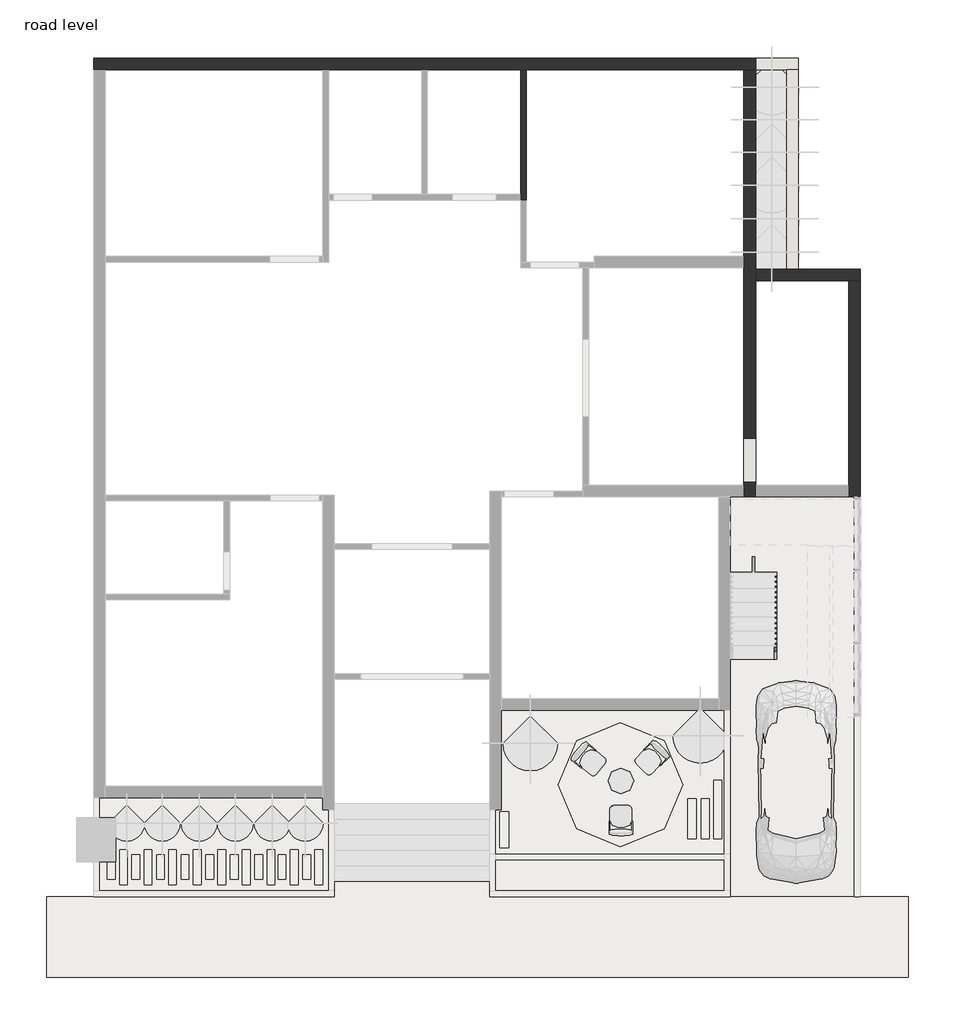
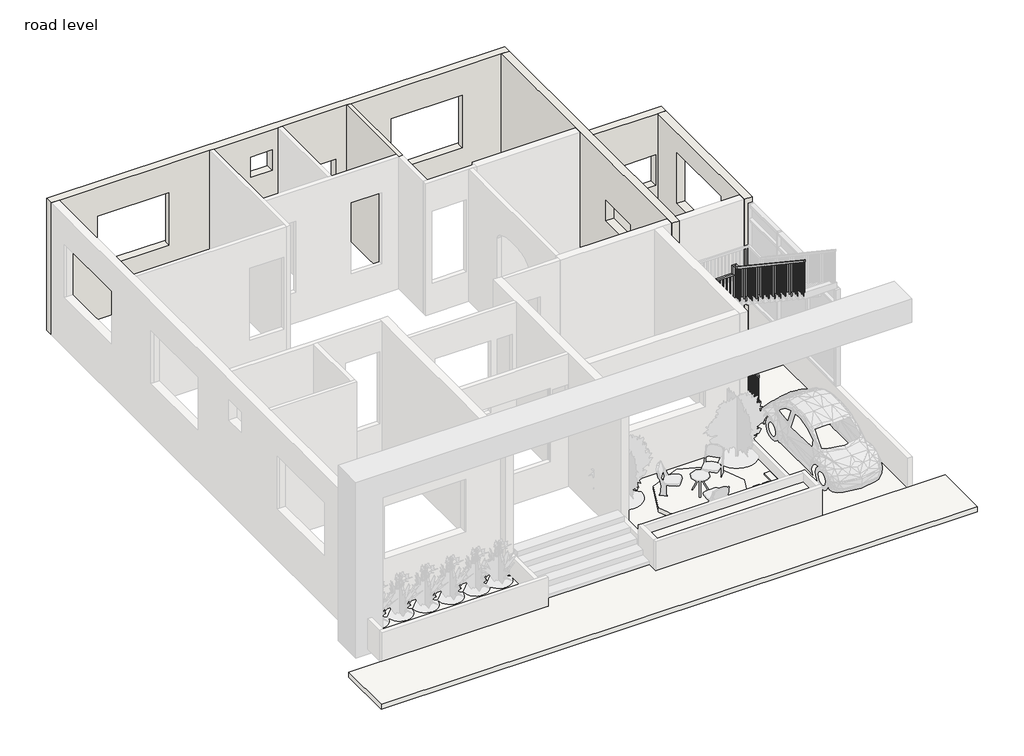
# One storey, part 2 of 3: 9 slabs, 7 walls, 1 railing.
"""IFC4 building model written with IfcOpenShell, lengths in millimetres."""

from ifc_helpers import new_model, si_unit, point, frame, frame_2d, origin, origin_with_axes, place, context, project, spatial, polyline, circle_curve, trimmed, segment, composite_curve, outline, extrude, faceted_brep, element, save

model = new_model("IFC4")

# Units and contexts
model_context = context("Model", 3, world=origin())
ifc_project = project(units=[si_unit("LENGTHUNIT", "METRE", prefix="MILLI")], contexts=[model_context])

# Site, building, storey
site = spatial("IfcSite", under=ifc_project)
building = spatial("IfcBuilding", under=site)
storey = spatial("IfcBuildingStorey", under=building, Name="road level", Elevation=0.0)

# Railing
placement = place(None, origin())
element("IfcRailing", 1, ObjectType="Handrail - Rectangular", at=placement, inside=storey, context=model_context, shape_type="SolidModel", body=[
    faceted_brep([(-6809.0994093, 3499.0237487, 1101.4363636), (-6809.0994093, 3499.0237487, 1040.3046237), (-6758.2994093, 3499.0237487, 1040.3046237), (-6758.2994093, 3499.0237487, 1101.4363636), (-6809.0994093, 5658.0237487, 2546.7173554), (-6809.0994093, 5708.8237487, 2519.592227), (-6758.2994093, 5708.8237487, 2519.592227), (-6758.2994093, 5658.0237487, 2546.7173554), (-6809.0994093, 5658.0237487, 2597.7272727), (-6809.0994093, 5708.8237487, 2546.9272727), (-6758.2994093, 5708.8237487, 2546.9272727), (-6758.2994093, 5658.0237487, 2597.7272727), (-6809.0994093, 5785.0237487, 2597.7272727), (-6809.0994093, 5785.0237487, 2546.9272727), (-6758.2994093, 5734.2237487, 2546.9272727), (-6758.2994093, 5734.2237487, 2597.7272727), (-6682.0994093, 5785.0237487, 2597.7272727), (-6682.0994093, 5785.0237487, 2546.9272727), (-6682.0994093, 5734.2237487, 2546.9272727), (-6682.0994093, 5734.2237487, 2597.7272727), (-6224.8994093, 5785.0237487, 2597.7272727), (-6174.0994093, 5785.0237487, 2546.9272727), (-6174.0994093, 5734.2237487, 2546.9272727), (-6224.8994093, 5734.2237487, 2597.7272727), (-6224.8994093, 5785.0237487, 2835.7735537), (-6174.0994093, 5785.0237487, 2784.9735537), (-6174.0994093, 5734.2237487, 2784.9735537), (-6224.8994093, 5734.2237487, 2835.7735537), (-6097.8994093, 5785.0237487, 2835.7735537), (-6097.8994093, 5785.0237487, 2784.9735537), (-6148.6994093, 5734.2237487, 2784.9735537), (-6148.6994093, 5734.2237487, 2835.7735537), (-6097.8994093, 5658.0237487, 2835.7735537), (-6097.8994093, 5642.5899149, 2784.9735537), (-6148.6994093, 5642.5899149, 2784.9735537), (-6148.6994093, 5658.0237487, 2835.7735537), (-6097.8994093, 2381.4237487, 5029.2), (-6148.6994093, 2381.4237487, 5029.2), (-6148.6994093, 2381.4237487, 4968.06826), (-6097.8994093, 2381.4237487, 4968.06826)], [[[0, 1, 2, 3]], [[1, 0, 4, 5]], [[2, 1, 5, 6]], [[3, 2, 6, 7]], [[0, 3, 7, 4]], [[5, 4, 8, 9]], [[6, 5, 9, 10]], [[7, 6, 10, 11]], [[4, 7, 11, 8]], [[9, 8, 12, 13]], [[10, 9, 13, 14]], [[11, 10, 14, 15]], [[8, 11, 15, 12]], [[13, 12, 16, 17]], [[14, 13, 17, 18]], [[15, 14, 18, 19]], [[12, 15, 19, 16]], [[17, 16, 20, 21]], [[18, 17, 21, 22]], [[19, 18, 22, 23]], [[16, 19, 23, 20]], [[21, 20, 24, 25]], [[22, 21, 25, 26]], [[23, 22, 26, 27]], [[20, 23, 27, 24]], [[25, 24, 28, 29]], [[26, 25, 29, 30]], [[27, 26, 30, 31]], [[24, 27, 31, 28]], [[29, 28, 32, 33]], [[30, 29, 33, 34]], [[31, 30, 34, 35]], [[28, 31, 35, 32]], [[36, 37, 38, 39]], [[33, 32, 36, 39]], [[34, 33, 39, 38]], [[35, 34, 38, 37]], [[32, 35, 37, 36]]]),
    extrude(outline(polyline([(2397.2987487, 4957.4411939), (2416.3487487, 4944.6887146), (2416.3487487, 3927.7636364), (2397.2987487, 3927.7636364), (2397.2987487, 4957.4411939)])), frame((-6132.8244093, 0.0, 0.0), z_axis=(1.0, 0.0, 0.0), x_axis=(0.0, 1.0, 0.0)), (0.0, 0.0, 1.0), 19.05),
    extrude(outline(polyline([(2498.8987487, 4889.4279708), (2517.9487487, 4876.6754914), (2517.9487487, 3927.7636364), (2498.8987487, 3927.7636364), (2498.8987487, 4889.4279708)])), frame((-6132.8244093, 0.0, 0.0), z_axis=(1.0, 0.0, 0.0), x_axis=(0.0, 1.0, 0.0)), (0.0, 0.0, 1.0), 19.05),
    extrude(outline(polyline([(2600.4987487, 4821.4147476), (2619.5487487, 4808.6622683), (2619.5487487, 3927.7636364), (2600.4987487, 3927.7636364), (2600.4987487, 4821.4147476)])), frame((-6132.8244093, 0.0, 0.0), z_axis=(1.0, 0.0, 0.0), x_axis=(0.0, 1.0, 0.0)), (0.0, 0.0, 1.0), 19.05),
    extrude(outline(polyline([(2702.0987487, 4753.4015245), (2721.1487487, 4740.6490452), (2721.1487487, 3740.7272727), (2702.0987487, 3740.7272727), (2702.0987487, 4753.4015245)])), frame((-6132.8244093, 0.0, 0.0), z_axis=(1.0, 0.0, 0.0), x_axis=(0.0, 1.0, 0.0)), (0.0, 0.0, 1.0), 19.05),
    extrude(outline(polyline([(2803.6987487, 4685.3883014), (2822.7487487, 4672.635822), (2822.7487487, 3740.7272727), (2803.6987487, 3740.7272727), (2803.6987487, 4685.3883014)])), frame((-6132.8244093, 0.0, 0.0), z_axis=(1.0, 0.0, 0.0), x_axis=(0.0, 1.0, 0.0)), (0.0, 0.0, 1.0), 19.05),
    extrude(outline(polyline([(2905.2987487, 4617.3750782), (2924.3487487, 4604.6225989), (2924.3487487, 3740.7272727), (2905.2987487, 3740.7272727), (2905.2987487, 4617.3750782)])), frame((-6132.8244093, 0.0, 0.0), z_axis=(1.0, 0.0, 0.0), x_axis=(0.0, 1.0, 0.0)), (0.0, 0.0, 1.0), 19.05),
    extrude(outline(polyline([(3006.8987487, 4549.3618551), (3025.9487487, 4536.6093757), (3025.9487487, 3553.6909091), (3006.8987487, 3553.6909091), (3006.8987487, 4549.3618551)])), frame((-6132.8244093, 0.0, 0.0), z_axis=(1.0, 0.0, 0.0), x_axis=(0.0, 1.0, 0.0)), (0.0, 0.0, 1.0), 19.05),
    extrude(outline(polyline([(3108.4987487, 4481.3486319), (3127.5487487, 4468.5961526), (3127.5487487, 3553.6909091), (3108.4987487, 3553.6909091), (3108.4987487, 4481.3486319)])), frame((-6132.8244093, 0.0, 0.0), z_axis=(1.0, 0.0, 0.0), x_axis=(0.0, 1.0, 0.0)), (0.0, 0.0, 1.0), 19.05),
    extrude(outline(polyline([(3210.0987487, 4413.3354088), (3229.1487487, 4400.5829295), (3229.1487487, 3553.6909091), (3210.0987487, 3553.6909091), (3210.0987487, 4413.3354088)])), frame((-6132.8244093, 0.0, 0.0), z_axis=(1.0, 0.0, 0.0), x_axis=(0.0, 1.0, 0.0)), (0.0, 0.0, 1.0), 19.05),
    extrude(outline(polyline([(3311.6987487, 4345.3221857), (3330.7487487, 4332.5697063), (3330.7487487, 3366.6545455), (3311.6987487, 3366.6545455), (3311.6987487, 4345.3221857)])), frame((-6132.8244093, 0.0, 0.0), z_axis=(1.0, 0.0, 0.0), x_axis=(0.0, 1.0, 0.0)), (0.0, 0.0, 1.0), 19.05),
    extrude(outline(polyline([(3413.2987487, 4277.3089625), (3432.3487487, 4264.5564832), (3432.3487487, 3366.6545455), (3413.2987487, 3366.6545455), (3413.2987487, 4277.3089625)])), frame((-6132.8244093, 0.0, 0.0), z_axis=(1.0, 0.0, 0.0), x_axis=(0.0, 1.0, 0.0)), (0.0, 0.0, 1.0), 19.05),
    extrude(outline(polyline([(3514.8987487, 4209.2957394), (3533.9487487, 4196.54326), (3533.9487487, 3179.6181818), (3514.8987487, 3179.6181818), (3514.8987487, 4209.2957394)])), frame((-6132.8244093, 0.0, 0.0), z_axis=(1.0, 0.0, 0.0), x_axis=(0.0, 1.0, 0.0)), (0.0, 0.0, 1.0), 19.05),
    extrude(outline(polyline([(3616.4987487, 4141.2825162), (3635.5487487, 4128.5300369), (3635.5487487, 3179.6181818), (3616.4987487, 3179.6181818), (3616.4987487, 4141.2825162)])), frame((-6132.8244093, 0.0, 0.0), z_axis=(1.0, 0.0, 0.0), x_axis=(0.0, 1.0, 0.0)), (0.0, 0.0, 1.0), 19.05),
    extrude(outline(polyline([(3718.0987487, 4073.2692931), (3737.1487487, 4060.5168138), (3737.1487487, 3179.6181818), (3718.0987487, 3179.6181818), (3718.0987487, 4073.2692931)])), frame((-6132.8244093, 0.0, 0.0), z_axis=(1.0, 0.0, 0.0), x_axis=(0.0, 1.0, 0.0)), (0.0, 0.0, 1.0), 19.05),
    extrude(outline(polyline([(3819.6987487, 4005.25607), (3838.7487487, 3992.5035906), (3838.7487487, 2992.5818182), (3819.6987487, 2992.5818182), (3819.6987487, 4005.25607)])), frame((-6132.8244093, 0.0, 0.0), z_axis=(1.0, 0.0, 0.0), x_axis=(0.0, 1.0, 0.0)), (0.0, 0.0, 1.0), 19.05),
    extrude(outline(polyline([(3921.2987487, 3937.2428468), (3940.3487487, 3924.4903675), (3940.3487487, 2992.5818182), (3921.2987487, 2992.5818182), (3921.2987487, 3937.2428468)])), frame((-6132.8244093, 0.0, 0.0), z_axis=(1.0, 0.0, 0.0), x_axis=(0.0, 1.0, 0.0)), (0.0, 0.0, 1.0), 19.05),
    extrude(outline(polyline([(4022.8987487, 3869.2296237), (4041.9487487, 3856.4771443), (4041.9487487, 2992.5818182), (4022.8987487, 2992.5818182), (4022.8987487, 3869.2296237)])), frame((-6132.8244093, 0.0, 0.0), z_axis=(1.0, 0.0, 0.0), x_axis=(0.0, 1.0, 0.0)), (0.0, 0.0, 1.0), 19.05),
    extrude(outline(polyline([(4124.4987487, 3801.2164005), (4143.5487487, 3788.4639212), (4143.5487487, 2805.5454545), (4124.4987487, 2805.5454545), (4124.4987487, 3801.2164005)])), frame((-6132.8244093, 0.0, 0.0), z_axis=(1.0, 0.0, 0.0), x_axis=(0.0, 1.0, 0.0)), (0.0, 0.0, 1.0), 19.05),
    extrude(outline(polyline([(4226.0987487, 3733.2031774), (4245.1487487, 3720.4506981), (4245.1487487, 2805.5454545), (4226.0987487, 2805.5454545), (4226.0987487, 3733.2031774)])), frame((-6132.8244093, 0.0, 0.0), z_axis=(1.0, 0.0, 0.0), x_axis=(0.0, 1.0, 0.0)), (0.0, 0.0, 1.0), 19.05),
    extrude(outline(polyline([(4327.6987487, 3665.1899543), (4346.7487487, 3652.4374749), (4346.7487487, 2805.5454545), (4327.6987487, 2805.5454545), (4327.6987487, 3665.1899543)])), frame((-6132.8244093, 0.0, 0.0), z_axis=(1.0, 0.0, 0.0), x_axis=(0.0, 1.0, 0.0)), (0.0, 0.0, 1.0), 19.05),
    extrude(outline(polyline([(4429.2987487, 3597.1767311), (4448.3487487, 3584.4242518), (4448.3487487, 2618.5090909), (4429.2987487, 2618.5090909), (4429.2987487, 3597.1767311)])), frame((-6132.8244093, 0.0, 0.0), z_axis=(1.0, 0.0, 0.0), x_axis=(0.0, 1.0, 0.0)), (0.0, 0.0, 1.0), 19.05),
    extrude(outline(polyline([(4530.8987487, 3529.163508), (4549.9487487, 3516.4110286), (4549.9487487, 2618.5090909), (4530.8987487, 2618.5090909), (4530.8987487, 3529.163508)])), frame((-6132.8244093, 0.0, 0.0), z_axis=(1.0, 0.0, 0.0), x_axis=(0.0, 1.0, 0.0)), (0.0, 0.0, 1.0), 19.05),
    extrude(outline(polyline([(4632.4987487, 3461.1502848), (4651.5487487, 3448.3978055), (4651.5487487, 2431.4727273), (4632.4987487, 2431.4727273), (4632.4987487, 3461.1502848)])), frame((-6132.8244093, 0.0, 0.0), z_axis=(1.0, 0.0, 0.0), x_axis=(0.0, 1.0, 0.0)), (0.0, 0.0, 1.0), 19.05),
    extrude(outline(polyline([(4734.0987487, 3393.1370617), (4753.1487487, 3380.3845824), (4753.1487487, 2431.4727273), (4734.0987487, 2431.4727273), (4734.0987487, 3393.1370617)])), frame((-6132.8244093, 0.0, 0.0), z_axis=(1.0, 0.0, 0.0), x_axis=(0.0, 1.0, 0.0)), (0.0, 0.0, 1.0), 19.05),
    extrude(outline(polyline([(4835.6987487, 3325.1238386), (4854.7487487, 3312.3713592), (4854.7487487, 2431.4727273), (4835.6987487, 2431.4727273), (4835.6987487, 3325.1238386)])), frame((-6132.8244093, 0.0, 0.0), z_axis=(1.0, 0.0, 0.0), x_axis=(0.0, 1.0, 0.0)), (0.0, 0.0, 1.0), 19.05),
    extrude(outline(polyline([(4937.2987487, 3257.1106154), (4956.3487487, 3244.3581361), (4956.3487487, 2244.4363636), (4937.2987487, 2244.4363636), (4937.2987487, 3257.1106154)])), frame((-6132.8244093, 0.0, 0.0), z_axis=(1.0, 0.0, 0.0), x_axis=(0.0, 1.0, 0.0)), (0.0, 0.0, 1.0), 19.05),
    extrude(outline(polyline([(5038.8987487, 3189.0973923), (5057.9487487, 3176.3449129), (5057.9487487, 2244.4363636), (5038.8987487, 2244.4363636), (5038.8987487, 3189.0973923)])), frame((-6132.8244093, 0.0, 0.0), z_axis=(1.0, 0.0, 0.0), x_axis=(0.0, 1.0, 0.0)), (0.0, 0.0, 1.0), 19.05),
    extrude(outline(polyline([(5140.4987487, 3121.0841691), (5159.5487487, 3108.3316898), (5159.5487487, 2244.4363636), (5140.4987487, 2244.4363636), (5140.4987487, 3121.0841691)])), frame((-6132.8244093, 0.0, 0.0), z_axis=(1.0, 0.0, 0.0), x_axis=(0.0, 1.0, 0.0)), (0.0, 0.0, 1.0), 19.05),
    extrude(outline(polyline([(5242.0987487, 3053.070946), (5261.1487487, 3040.3184667), (5261.1487487, 2057.4), (5242.0987487, 2057.4), (5242.0987487, 3053.070946)])), frame((-6132.8244093, 0.0, 0.0), z_axis=(1.0, 0.0, 0.0), x_axis=(0.0, 1.0, 0.0)), (0.0, 0.0, 1.0), 19.05),
    extrude(outline(polyline([(5343.6987487, 2985.0577229), (5362.7487487, 2972.3052435), (5362.7487487, 2057.4), (5343.6987487, 2057.4), (5343.6987487, 2985.0577229)])), frame((-6132.8244093, 0.0, 0.0), z_axis=(1.0, 0.0, 0.0), x_axis=(0.0, 1.0, 0.0)), (0.0, 0.0, 1.0), 19.05),
    extrude(outline(polyline([(5445.2987487, 2917.0444997), (5464.3487487, 2904.2920204), (5464.3487487, 2057.4), (5445.2987487, 2057.4), (5445.2987487, 2917.0444997)])), frame((-6132.8244093, 0.0, 0.0), z_axis=(1.0, 0.0, 0.0), x_axis=(0.0, 1.0, 0.0)), (0.0, 0.0, 1.0), 19.05),
    extrude(outline(polyline([(5546.8987487, 2849.0312766), (5565.9487487, 2836.2787972), (5565.9487487, 1870.3636364), (5546.8987487, 1870.3636364), (5546.8987487, 2849.0312766)])), frame((-6132.8244093, 0.0, 0.0), z_axis=(1.0, 0.0, 0.0), x_axis=(0.0, 1.0, 0.0)), (0.0, 0.0, 1.0), 19.05),
    extrude(outline(polyline([(5648.4987487, 2781.0180534), (5667.5487487, 2768.2655741), (5667.5487487, 1870.3636364), (5648.4987487, 1870.3636364), (5648.4987487, 2781.0180534)])), frame((-6132.8244093, 0.0, 0.0), z_axis=(1.0, 0.0, 0.0), x_axis=(0.0, 1.0, 0.0)), (0.0, 0.0, 1.0), 19.05),
    extrude(outline(polyline([(-6183.6244093, 5750.0987487), (-6183.6244093, 5769.1487487), (-6164.5744093, 5769.1487487), (-6164.5744093, 5750.0987487), (-6183.6244093, 5750.0987487)])), frame((0.0, 0.0, 1683.3272727), z_axis=(0.0, 0.0, 1.0), x_axis=(1.0, 0.0, 0.0)), (0.0, 0.0, 1.0), 1101.646281),
    extrude(outline(polyline([(-6285.2244093, 5750.0987487), (-6285.2244093, 5769.1487487), (-6266.1744093, 5769.1487487), (-6266.1744093, 5750.0987487), (-6285.2244093, 5750.0987487)])), frame((0.0, 0.0, 1683.3272727), z_axis=(0.0, 0.0, 1.0), x_axis=(1.0, 0.0, 0.0)), (0.0, 0.0, 1.0), 863.6),
    extrude(outline(polyline([(-6386.8244093, 5750.0987487), (-6386.8244093, 5769.1487487), (-6367.7744093, 5769.1487487), (-6367.7744093, 5750.0987487), (-6386.8244093, 5750.0987487)])), frame((0.0, 0.0, 1683.3272727), z_axis=(0.0, 0.0, 1.0), x_axis=(1.0, 0.0, 0.0)), (0.0, 0.0, 1.0), 863.6),
    extrude(outline(polyline([(-6488.4244093, 5750.0987487), (-6488.4244093, 5769.1487487), (-6469.3744093, 5769.1487487), (-6469.3744093, 5750.0987487), (-6488.4244093, 5750.0987487)])), frame((0.0, 0.0, 1683.3272727), z_axis=(0.0, 0.0, 1.0), x_axis=(1.0, 0.0, 0.0)), (0.0, 0.0, 1.0), 863.6),
    extrude(outline(polyline([(-6590.0244093, 5750.0987487), (-6590.0244093, 5769.1487487), (-6570.9744093, 5769.1487487), (-6570.9744093, 5750.0987487), (-6590.0244093, 5750.0987487)])), frame((0.0, 0.0, 1683.3272727), z_axis=(0.0, 0.0, 1.0), x_axis=(1.0, 0.0, 0.0)), (0.0, 0.0, 1.0), 863.6),
    extrude(outline(polyline([(-6691.6244093, 5750.0987487), (-6691.6244093, 5769.1487487), (-6672.5744093, 5769.1487487), (-6672.5744093, 5750.0987487), (-6691.6244093, 5750.0987487)])), frame((0.0, 0.0, 1683.3272727), z_axis=(0.0, 0.0, 1.0), x_axis=(1.0, 0.0, 0.0)), (0.0, 0.0, 1.0), 863.6),
    extrude(outline(polyline([(-6774.1744093, 5724.6987487), (-6793.2244093, 5724.6987487), (-6793.2244093, 5743.7487487), (-6774.1744093, 5743.7487487), (-6774.1744093, 5724.6987487)])), frame((0.0, 0.0, 1683.3272727), z_axis=(0.0, 0.0, 1.0), x_axis=(1.0, 0.0, 0.0)), (0.0, 0.0, 1.0), 863.6),
    extrude(outline(polyline([(5623.0987487, 2462.20607), (5642.1487487, 2474.9585493), (5642.1487487, 1496.2909091), (5623.0987487, 1496.2909091), (5623.0987487, 2462.20607)])), frame((-6793.2244093, 0.0, 0.0), z_axis=(1.0, 0.0, 0.0), x_axis=(0.0, 1.0, 0.0)), (0.0, 0.0, 1.0), 19.05),
    extrude(outline(polyline([(5521.4987487, 2394.1928468), (5540.5487487, 2406.9453262), (5540.5487487, 1496.2909091), (5521.4987487, 1496.2909091), (5521.4987487, 2394.1928468)])), frame((-6793.2244093, 0.0, 0.0), z_axis=(1.0, 0.0, 0.0), x_axis=(0.0, 1.0, 0.0)), (0.0, 0.0, 1.0), 19.05),
    extrude(outline(polyline([(5419.8987487, 2326.1796237), (5438.9487487, 2338.932103), (5438.9487487, 1309.2545455), (5419.8987487, 1309.2545455), (5419.8987487, 2326.1796237)])), frame((-6793.2244093, 0.0, 0.0), z_axis=(1.0, 0.0, 0.0), x_axis=(0.0, 1.0, 0.0)), (0.0, 0.0, 1.0), 19.05),
    extrude(outline(polyline([(5318.2987487, 2258.1664005), (5337.3487487, 2270.9188799), (5337.3487487, 1309.2545455), (5318.2987487, 1309.2545455), (5318.2987487, 2258.1664005)])), frame((-6793.2244093, 0.0, 0.0), z_axis=(1.0, 0.0, 0.0), x_axis=(0.0, 1.0, 0.0)), (0.0, 0.0, 1.0), 19.05),
    extrude(outline(polyline([(5216.6987487, 2190.1531774), (5235.7487487, 2202.9056567), (5235.7487487, 1309.2545455), (5216.6987487, 1309.2545455), (5216.6987487, 2190.1531774)])), frame((-6793.2244093, 0.0, 0.0), z_axis=(1.0, 0.0, 0.0), x_axis=(0.0, 1.0, 0.0)), (0.0, 0.0, 1.0), 19.05),
    extrude(outline(polyline([(5115.0987487, 2122.1399543), (5134.1487487, 2134.8924336), (5134.1487487, 1122.2181818), (5115.0987487, 1122.2181818), (5115.0987487, 2122.1399543)])), frame((-6793.2244093, 0.0, 0.0), z_axis=(1.0, 0.0, 0.0), x_axis=(0.0, 1.0, 0.0)), (0.0, 0.0, 1.0), 19.05),
    extrude(outline(polyline([(5013.4987487, 2054.1267311), (5032.5487487, 2066.8792105), (5032.5487487, 1122.2181818), (5013.4987487, 1122.2181818), (5013.4987487, 2054.1267311)])), frame((-6793.2244093, 0.0, 0.0), z_axis=(1.0, 0.0, 0.0), x_axis=(0.0, 1.0, 0.0)), (0.0, 0.0, 1.0), 19.05),
    extrude(outline(polyline([(4911.8987487, 1986.113508), (4930.9487487, 1998.8659873), (4930.9487487, 1122.2181818), (4911.8987487, 1122.2181818), (4911.8987487, 1986.113508)])), frame((-6793.2244093, 0.0, 0.0), z_axis=(1.0, 0.0, 0.0), x_axis=(0.0, 1.0, 0.0)), (0.0, 0.0, 1.0), 19.05),
    extrude(outline(polyline([(4810.2987487, 1918.1002848), (4829.3487487, 1930.8527642), (4829.3487487, 935.1818182), (4810.2987487, 935.1818182), (4810.2987487, 1918.1002848)])), frame((-6793.2244093, 0.0, 0.0), z_axis=(1.0, 0.0, 0.0), x_axis=(0.0, 1.0, 0.0)), (0.0, 0.0, 1.0), 19.05),
    extrude(outline(polyline([(4708.6987487, 1850.0870617), (4727.7487487, 1862.839541), (4727.7487487, 935.1818182), (4708.6987487, 935.1818182), (4708.6987487, 1850.0870617)])), frame((-6793.2244093, 0.0, 0.0), z_axis=(1.0, 0.0, 0.0), x_axis=(0.0, 1.0, 0.0)), (0.0, 0.0, 1.0), 19.05),
    extrude(outline(polyline([(4607.0987487, 1782.0738386), (4626.1487487, 1794.8263179), (4626.1487487, 935.1818182), (4607.0987487, 935.1818182), (4607.0987487, 1782.0738386)])), frame((-6793.2244093, 0.0, 0.0), z_axis=(1.0, 0.0, 0.0), x_axis=(0.0, 1.0, 0.0)), (0.0, 0.0, 1.0), 19.05),
    extrude(outline(polyline([(4505.4987487, 1714.0606154), (4524.5487487, 1726.8130948), (4524.5487487, 748.1454545), (4505.4987487, 748.1454545), (4505.4987487, 1714.0606154)])), frame((-6793.2244093, 0.0, 0.0), z_axis=(1.0, 0.0, 0.0), x_axis=(0.0, 1.0, 0.0)), (0.0, 0.0, 1.0), 19.05),
    extrude(outline(polyline([(4403.8987487, 1646.0473923), (4422.9487487, 1658.7998716), (4422.9487487, 748.1454545), (4403.8987487, 748.1454545), (4403.8987487, 1646.0473923)])), frame((-6793.2244093, 0.0, 0.0), z_axis=(1.0, 0.0, 0.0), x_axis=(0.0, 1.0, 0.0)), (0.0, 0.0, 1.0), 19.05),
    extrude(outline(polyline([(4302.2987487, 1578.0341691), (4321.3487487, 1590.7866485), (4321.3487487, 561.1090909), (4302.2987487, 561.1090909), (4302.2987487, 1578.0341691)])), frame((-6793.2244093, 0.0, 0.0), z_axis=(1.0, 0.0, 0.0), x_axis=(0.0, 1.0, 0.0)), (0.0, 0.0, 1.0), 19.05),
    extrude(outline(polyline([(4200.6987487, 1510.020946), (4219.7487487, 1522.7734253), (4219.7487487, 561.1090909), (4200.6987487, 561.1090909), (4200.6987487, 1510.020946)])), frame((-6793.2244093, 0.0, 0.0), z_axis=(1.0, 0.0, 0.0), x_axis=(0.0, 1.0, 0.0)), (0.0, 0.0, 1.0), 19.05),
    extrude(outline(polyline([(4099.0987487, 1442.0077229), (4118.1487487, 1454.7602022), (4118.1487487, 561.1090909), (4099.0987487, 561.1090909), (4099.0987487, 1442.0077229)])), frame((-6793.2244093, 0.0, 0.0), z_axis=(1.0, 0.0, 0.0), x_axis=(0.0, 1.0, 0.0)), (0.0, 0.0, 1.0), 19.05),
    extrude(outline(polyline([(3997.4987487, 1373.9944997), (4016.5487487, 1386.746979), (4016.5487487, 374.0727273), (3997.4987487, 374.0727273), (3997.4987487, 1373.9944997)])), frame((-6793.2244093, 0.0, 0.0), z_axis=(1.0, 0.0, 0.0), x_axis=(0.0, 1.0, 0.0)), (0.0, 0.0, 1.0), 19.05),
    extrude(outline(polyline([(3895.8987487, 1305.9812766), (3914.9487487, 1318.7337559), (3914.9487487, 374.0727273), (3895.8987487, 374.0727273), (3895.8987487, 1305.9812766)])), frame((-6793.2244093, 0.0, 0.0), z_axis=(1.0, 0.0, 0.0), x_axis=(0.0, 1.0, 0.0)), (0.0, 0.0, 1.0), 19.05),
    extrude(outline(polyline([(3794.2987487, 1237.9680534), (3813.3487487, 1250.7205328), (3813.3487487, 374.0727273), (3794.2987487, 374.0727273), (3794.2987487, 1237.9680534)])), frame((-6793.2244093, 0.0, 0.0), z_axis=(1.0, 0.0, 0.0), x_axis=(0.0, 1.0, 0.0)), (0.0, 0.0, 1.0), 19.05),
    extrude(outline(polyline([(3692.6987487, 1169.9548303), (3711.7487487, 1182.7073096), (3711.7487487, 187.0363636), (3692.6987487, 187.0363636), (3692.6987487, 1169.9548303)])), frame((-6793.2244093, 0.0, 0.0), z_axis=(1.0, 0.0, 0.0), x_axis=(0.0, 1.0, 0.0)), (0.0, 0.0, 1.0), 19.05),
    extrude(outline(polyline([(3591.0987487, 1101.9416071), (3610.1487487, 1114.6940865), (3610.1487487, 187.0363636), (3591.0987487, 187.0363636), (3591.0987487, 1101.9416071)])), frame((-6793.2244093, 0.0, 0.0), z_axis=(1.0, 0.0, 0.0), x_axis=(0.0, 1.0, 0.0)), (0.0, 0.0, 1.0), 19.05),
    extrude(outline(polyline([(-6132.8244093, 5750.0987487), (-6132.8244093, 5769.1487487), (-6113.7744093, 5769.1487487), (-6113.7744093, 5750.0987487), (-6132.8244093, 5750.0987487)])), frame((0.0, 0.0, 1683.3272727), z_axis=(0.0, 0.0, 1.0), x_axis=(1.0, 0.0, 0.0)), (0.0, 0.0, 1.0), 1101.646281),
    extrude(outline(polyline([(-6774.1744093, 5750.0987487), (-6793.2244093, 5750.0987487), (-6793.2244093, 5769.1487487), (-6774.1744093, 5769.1487487), (-6774.1744093, 5750.0987487)])), frame((0.0, 0.0, 1683.3272727), z_axis=(0.0, 0.0, 1.0), x_axis=(1.0, 0.0, 0.0)), (0.0, 0.0, 1.0), 863.6),
    extrude(outline(polyline([(2381.4237487, 4968.06826), (2400.4737487, 4955.3157807), (2400.4737487, 3927.7636364), (2381.4237487, 3927.7636364), (2381.4237487, 4968.06826)])), frame((-6132.8244093, 0.0, 0.0), z_axis=(1.0, 0.0, 0.0), x_axis=(0.0, 1.0, 0.0)), (0.0, 0.0, 1.0), 19.05),
    extrude(outline(polyline([(3499.0237487, 1040.3046237), (3518.0737487, 1053.057103), (3518.0737487, 187.0363636), (3499.0237487, 187.0363636), (3499.0237487, 1040.3046237)])), frame((-6793.2244093, 0.0, 0.0), z_axis=(1.0, 0.0, 0.0), x_axis=(0.0, 1.0, 0.0)), (0.0, 0.0, 1.0), 19.05),
])

# Slabs
element("IfcSlab", 2, ObjectType="Generic - 2\"", at=placement, inside=storey, context=model_context, shape_type="SweptSolid", body=[
    extrude(outline(polyline([(-15826.0994093, -240.581619), (-15673.6994093, -240.581619), (-15673.6994093, -926.381619), (-15826.0994093, -926.381619), (-15826.0994093, -240.581619)])), origin_with_axes(), (0.0, 0.0, 1.0), 50.8),
    extrude(outline(polyline([(-16064.1206657, -338.9515207), (-15911.7206657, -338.9515207), (-15911.7206657, -821.5515207), (-16064.1206657, -821.5515207), (-16064.1206657, -338.9515207)])), origin_with_axes(), (0.0, 0.0, 1.0), 50.8),
    extrude(outline(polyline([(-16156.2994093, -926.381619), (-16308.6994093, -926.381619), (-16308.6994093, -240.581619), (-16156.2994093, -240.581619), (-16156.2994093, -926.381619)])), origin_with_axes(), (0.0, 0.0, 1.0), 50.8),
    extrude(outline(polyline([(-16546.7206657, -338.9515207), (-16394.3206657, -338.9515207), (-16394.3206657, -821.5515207), (-16546.7206657, -821.5515207), (-16546.7206657, -338.9515207)])), origin_with_axes(), (0.0, 0.0, 1.0), 50.8),
    extrude(outline(polyline([(-16765.8994093, -240.581619), (-16613.4994093, -240.581619), (-16613.4994093, -926.381619), (-16765.8994093, -926.381619), (-16765.8994093, -240.581619)])), origin_with_axes(), (0.0, 0.0, 1.0), 50.8),
    extrude(outline(polyline([(-17003.9206657, -338.9515207), (-16851.5206657, -338.9515207), (-16851.5206657, -821.5515207), (-17003.9206657, -821.5515207), (-17003.9206657, -338.9515207)])), origin_with_axes(), (0.0, 0.0, 1.0), 50.8),
    extrude(outline(polyline([(-17248.4994093, -240.581619), (-17096.0994093, -240.581619), (-17096.0994093, -926.381619), (-17248.4994093, -926.381619), (-17248.4994093, -240.581619)])), origin_with_axes(), (0.0, 0.0, 1.0), 50.8),
    extrude(outline(polyline([(-17486.5206657, -338.9515207), (-17334.1206657, -338.9515207), (-17334.1206657, -821.5515207), (-17486.5206657, -821.5515207), (-17486.5206657, -338.9515207)])), origin_with_axes(), (0.0, 0.0, 1.0), 50.8),
    extrude(outline(polyline([(-17731.0994093, -240.581619), (-17578.6994093, -240.581619), (-17578.6994093, -926.381619), (-17731.0994093, -926.381619), (-17731.0994093, -240.581619)])), origin_with_axes(), (0.0, 0.0, 1.0), 50.8),
    extrude(outline(polyline([(-17969.1206657, -338.9515207), (-17816.7206657, -338.9515207), (-17816.7206657, -821.5515207), (-17969.1206657, -821.5515207), (-17969.1206657, -338.9515207)])), origin_with_axes(), (0.0, 0.0, 1.0), 50.8),
    extrude(outline(polyline([(-18213.6994093, -240.581619), (-18061.2994093, -240.581619), (-18061.2994093, -926.381619), (-18213.6994093, -926.381619), (-18213.6994093, -240.581619)])), origin_with_axes(), (0.0, 0.0, 1.0), 50.8),
    extrude(outline(polyline([(-18451.7206657, -338.9515207), (-18299.3206657, -338.9515207), (-18299.3206657, -821.5515207), (-18451.7206657, -821.5515207), (-18451.7206657, -338.9515207)])), origin_with_axes(), (0.0, 0.0, 1.0), 50.8),
    extrude(outline(polyline([(-18543.8994093, -926.381619), (-18696.2994093, -926.381619), (-18696.2994093, -240.581619), (-18543.8994093, -240.581619), (-18543.8994093, -926.381619)])), origin_with_axes(), (0.0, 0.0, 1.0), 50.8),
    extrude(outline(polyline([(-18934.3206657, -338.9515207), (-18781.9206657, -338.9515207), (-18781.9206657, -821.5515207), (-18934.3206657, -821.5515207), (-18934.3206657, -338.9515207)])), origin_with_axes(), (0.0, 0.0, 1.0), 50.8),
    extrude(outline(polyline([(-19026.4994093, -926.381619), (-19178.8994093, -926.381619), (-19178.8994093, -240.581619), (-19026.4994093, -240.581619), (-19026.4994093, -926.381619)])), origin_with_axes(), (0.0, 0.0, 1.0), 50.8),
    extrude(outline(polyline([(-19416.9206657, -338.9515207), (-19264.5206657, -338.9515207), (-19264.5206657, -821.5515207), (-19416.9206657, -821.5515207), (-19416.9206657, -338.9515207)])), origin_with_axes(), (0.0, 0.0, 1.0), 50.8),
    extrude(outline(polyline([(-19661.4994093, -926.381619), (-19661.4994093, -240.581619), (-19509.0994093, -240.581619), (-19509.0994093, -926.381619), (-19661.4994093, -926.381619)])), origin_with_axes(), (0.0, 0.0, 1.0), 50.8),
    extrude(outline(polyline([(-19899.5206657, -338.9515207), (-19747.1206657, -338.9515207), (-19747.1206657, -821.5515207), (-19899.5206657, -821.5515207), (-19899.5206657, -338.9515207)])), origin_with_axes(), (0.0, 0.0, 1.0), 50.8),
])
element("IfcSlab", 3, ObjectType="Generic - 2\"", at=placement, inside=storey, context=model_context, shape_type="SweptSolid", body=[
    extrude(outline(polyline([(-7994.8454717, 1123.7453596), (-7842.4454717, 1123.7453596), (-7842.4454717, -19.2546404), (-7994.8454717, -19.2546404), (-7994.8454717, 1123.7453596)])), origin_with_axes(), (0.0, 0.0, 1.0), 50.8),
    extrude(outline(polyline([(-8247.1172864, 766.6361768), (-8086.9279122, 766.6361768), (-8086.9279122, -19.2546404), (-8247.1172864, -19.2546404), (-8247.1172864, 766.6361768)])), origin_with_axes(), (0.0, 0.0, 1.0), 50.8),
    extrude(outline(polyline([(-8510.0405442, 766.6361768), (-8345.1453213, 766.6361768), (-8345.1453213, -19.2546404), (-8510.0405442, -19.2546404), (-8510.0405442, 766.6361768)])), origin_with_axes(), (0.0, 0.0, 1.0), 50.8),
    extrude(outline(polyline([(-12198.4229103, 508.4187677), (-12020.6229103, 508.4187677), (-12020.6229103, -202.7812323), (-12198.4229103, -202.7812323), (-12198.4229103, 508.4187677)])), origin_with_axes(), (0.0, 0.0, 1.0), 50.8),
])
element("IfcSlab", 4, ObjectType="Generic - 4\"", at=placement, inside=storey, context=model_context, shape_type="SweptSolid", body=[
    extrude(outline(polyline([(-7786.9996518, -438.0872312), (-7786.9996518, -1047.6872312), (-12282.7996518, -1047.6872312), (-12282.7996518, -438.0872312), (-7786.9996518, -438.0872312)])), origin_with_axes(), (0.0, 0.0, 1.0), 609.6),
])
element("IfcSlab", 5, ObjectType="Generic - 4\" 2 2\"", at=placement, inside=storey, context=model_context, shape_type="SweptSolid", body=[
    extrude(outline(polyline([(-7786.9994093, -437.9762513), (-7786.9994093, -1047.5762513), (-12282.7994093, -1047.5762513), (-12282.7994093, -437.9762513), (-7786.9994093, -437.9762513)])), frame((0.0, 0.0, 609.6), z_axis=(0.0, 0.0, 1.0), x_axis=(1.0, 0.0, 0.0)), (0.0, 0.0, 1.0), 50.8),
])
element("IfcSlab", 6, ObjectType="Generic - 6\" -2", at=placement, inside=storey, context=model_context, shape_type="SweptSolid", body=[
    extrude(outline(polyline([(-20055.1994093, -1047.5762513), (-20055.1994093, 781.2237487), (-15673.6994093, 781.2237487), (-15673.6994093, 546.2737487), (-15559.3994093, 546.2737487), (-15559.3994093, -1047.5762513), (-20055.1994093, -1047.5762513)])), frame((0.0, 0.0, -152.4), z_axis=(0.0, 0.0, 1.0), x_axis=(1.0, 0.0, 0.0)), (0.0, 0.0, 1.0), 152.4),
    extrude(outline(polyline([(-12168.4994093, 2495.7237487), (-7786.9994093, 2495.7237487), (-7786.9994093, -323.6762513), (-12282.7994093, -323.6762513), (-12282.7994093, 546.2737487), (-12168.4994093, 546.2737487), (-12168.4994093, 2495.7237487)])), frame((0.0, 0.0, -152.4), z_axis=(0.0, 0.0, 1.0), x_axis=(1.0, 0.0, 0.0)), (0.0, 0.0, 1.0), 152.4),
])
element("IfcSlab", 7, ObjectType="Generic - 6\" -3", at=placement, inside=storey, context=model_context, shape_type="SweptSolid", body=[
    extrude(outline(polyline([(-5119.9994093, 6686.7237487), (-5119.9994093, -1161.8762513), (-7672.6994093, -1161.8762513), (-7672.6994093, 6686.7237487), (-5119.9994093, 6686.7237487)])), frame((0.0, 0.0, -152.4), z_axis=(0.0, 0.0, 1.0), x_axis=(1.0, 0.0, 0.0)), (0.0, 0.0, 1.0), 152.4),
])
element("IfcSlab", 8, ObjectType="Generic - 6\" -3 2", at=placement, inside=storey, context=model_context, shape_type="SweptSolid", body=[
    extrude(outline(polyline([(-6567.7994093, 15068.7237487), (-6567.7994093, 11157.1237487), (-7177.3994093, 11157.1237487), (-7177.3994093, 15068.7237487), (-6567.7994093, 15068.7237487)])), frame((0.0, 0.0, -152.4), z_axis=(0.0, 0.0, 1.0), x_axis=(1.0, 0.0, 0.0)), (0.0, 0.0, 1.0), 152.4),
])
element("IfcSlab", 9, ObjectType="Generic - 6\" -4", at=placement, inside=storey, context=model_context, shape_type="SweptSolid", body=[
    extrude(outline(composite_curve([segment(trimmed(circle_curve(frame_2d((-9828.4647361, 1035.6591175)), 1218.556629), [point((-11047.0213652, 1035.6591175))], [point((-8609.9081071, 1035.6591175))], False, "CARTESIAN"), True, "CONTINUOUS"), segment(trimmed(circle_curve(frame_2d((-9828.4647361, 1035.6591175)), 1218.556629), [point((-8609.9081071, 1035.6591175))], [point((-11047.0213652, 1035.6591175))], False, "CARTESIAN"), True, "CONTINUOUS")], self_intersect=False)), frame((0.0, 0.0, -25.4), z_axis=(0.0, 0.0, 1.0), x_axis=(1.0, 0.0, 0.0)), (0.0, 0.0, 1.0), 152.4),
])
element("IfcSlab", 10, ObjectType="Generic - 6\" 7", at=placement, inside=storey, context=model_context, shape_type="SweptSolid", body=[
    extrude(outline(polyline([(-21094.2265318, -1161.8762513), (-17299.2994093, -1161.8762513), (-15445.0994093, -1161.8762513), (-15445.0994093, -857.0762513), (-12397.0994093, -857.0762513), (-12397.0994093, -1161.8762513), (-4177.8265318, -1161.8762513), (-4177.8265318, -2744.8172329), (-21094.2265318, -2744.8172329), (-21094.2265318, -1161.8762513)])), frame((0.0, 0.0, -101.6), z_axis=(0.0, 0.0, 1.0), x_axis=(1.0, 0.0, 0.0)), (0.0, 0.0, 1.0), 152.4),
])

# Walls
element("IfcWall", 11, ObjectType="Generic - 4.5\"", at=placement, inside=storey, context=model_context, shape_type="Brep", body=[
    faceted_brep([(-11787.4994093, 15068.7237487, 0.0), (-11787.4994093, 12630.3237487, 0.0), (-11787.4994093, 12516.0237487, 0.0), (-11787.4994093, 12516.0237487, 3962.4), (-11787.4994093, 12630.3237487, 3962.4), (-11787.4994093, 15068.7237487, 3962.4), (-11673.1994093, 15068.7237487, 0.0), (-11673.1994093, 15068.7237487, 3962.4), (-11673.1994093, 12516.0237487, 3962.4), (-11673.1994093, 12516.0237487, 0.0)], [[[0, 1, 2, 3, 4, 5]], [[6, 7, 8, 9]], [[2, 1, 0, 6, 9]], [[0, 5, 7, 6]], [[3, 2, 9, 8]], [[5, 4, 3, 8, 7]]]),
])
element("IfcWall", 12, ObjectType="Generic - 9\"", at=placement, inside=storey, context=model_context, shape_type="Brep", body=[
    faceted_brep([(-20169.4994093, 15068.7237487, 0.0), (-19940.8994093, 15068.7237487, 0.0), (-15673.6994093, 15068.7237487, 0.0), (-15559.3994093, 15068.7237487, 0.0), (-13730.5994093, 15068.7237487, 0.0), (-13616.2994093, 15068.7237487, 0.0), (-11787.4994093, 15068.7237487, 0.0), (-11673.1994093, 15068.7237487, 0.0), (-7405.9994093, 15068.7237487, 0.0), (-7291.6994093, 15068.7237487, 0.0), (-7291.6994093, 15068.7237487, 914.4), (-7177.3994093, 15068.7237487, 914.4), (-7177.3994093, 15068.7237487, 3962.4), (-7405.9994093, 15068.7237487, 3962.4), (-11673.1994093, 15068.7237487, 3962.4), (-11787.4994093, 15068.7237487, 3962.4), (-13616.2994093, 15068.7237487, 3962.4), (-13730.5994093, 15068.7237487, 3962.4), (-15559.3994093, 15068.7237487, 3962.4), (-15673.6994093, 15068.7237487, 3962.4), (-19940.8994093, 15068.7237487, 3962.4), (-20169.4994093, 15068.7237487, 3962.4), (-18843.0578862, 15068.7237487, 3098.8), (-16828.6909324, 15068.7237487, 3098.8), (-16828.6909324, 15068.7237487, 1524.0), (-18843.0578862, 15068.7237487, 1524.0), (-10518.2078862, 15068.7237487, 3098.8), (-8503.8409324, 15068.7237487, 3098.8), (-8503.8409324, 15068.7237487, 1524.0), (-10518.2078862, 15068.7237487, 1524.0), (-12092.2994093, 15068.7237487, 2438.4), (-12092.2994093, 15068.7237487, 1828.8), (-13311.4994093, 15068.7237487, 1828.8), (-13311.4994093, 15068.7237487, 2438.4), (-14511.6494093, 15068.7237487, 3352.8), (-13902.0494093, 15068.7237487, 3352.8), (-13902.0494093, 15068.7237487, 2743.2), (-14511.6494093, 15068.7237487, 2743.2), (-20169.4994093, 15297.3237487, 0.0), (-20169.4994093, 15297.3237487, 3962.4), (-7177.3994093, 15297.3237487, 3962.4), (-7177.3994093, 15297.3237487, 914.4), (-7291.6994093, 15297.3237487, 914.4), (-7291.6994093, 15297.3237487, 0.0), (-16793.7659324, 15297.3237487, 3098.8), (-18877.9828862, 15297.3237487, 3098.8), (-18877.9828862, 15297.3237487, 1524.0), (-16793.7659324, 15297.3237487, 1524.0), (-8468.9159324, 15297.3237487, 3098.8), (-10553.1328862, 15297.3237487, 3098.8), (-10553.1328862, 15297.3237487, 1524.0), (-8468.9159324, 15297.3237487, 1524.0), (-12092.2994093, 15297.3237487, 2438.4), (-13311.4994093, 15297.3237487, 2438.4), (-13311.4994093, 15297.3237487, 1828.8), (-12092.2994093, 15297.3237487, 1828.8), (-14511.6494093, 15297.3237487, 3352.8), (-14511.6494093, 15297.3237487, 2743.2), (-13902.0494093, 15297.3237487, 2743.2), (-13902.0494093, 15297.3237487, 3352.8), (-18843.0578862, 15236.8318742, 3098.8), (-16828.6909324, 15236.8318742, 3098.8), (-18843.0578862, 15236.8318742, 1524.0), (-16828.6909324, 15236.8318742, 1524.0), (-10518.2078862, 15236.8318742, 3098.8), (-8503.8409324, 15236.8318742, 3098.8), (-10518.2078862, 15236.8318742, 1524.0), (-8503.8409324, 15236.8318742, 1524.0)], [[[0, 1, 2, 3, 4, 5, 6, 7, 8, 9, 10, 11, 12, 13, 14, 15, 16, 17, 18, 19, 20, 21], [22, 23, 24, 25], [26, 27, 28, 29], [30, 31, 32, 33], [34, 35, 36, 37]], [[38, 39, 40, 41, 42, 43], [44, 45, 46, 47], [48, 49, 50, 51], [52, 53, 54, 55], [56, 57, 58, 59]], [[9, 8, 7, 6, 5, 4, 3, 2, 1, 0, 38, 43]], [[0, 21, 39, 38]], [[60, 45, 44, 61, 23, 22]], [[62, 25, 24, 63, 47, 46]], [[60, 22, 25, 62]], [[23, 61, 63, 24]], [[61, 44, 47, 63]], [[45, 60, 62, 46]], [[64, 49, 48, 65, 27, 26]], [[66, 29, 28, 67, 51, 50]], [[64, 26, 29, 66]], [[27, 65, 67, 28]], [[65, 48, 51, 67]], [[49, 64, 66, 50]], [[31, 30, 52, 55]], [[32, 31, 55, 54]], [[33, 32, 54, 53]], [[30, 33, 53, 52]], [[57, 56, 34, 37]], [[58, 57, 37, 36]], [[59, 58, 36, 35]], [[56, 59, 35, 34]], [[10, 9, 43, 42]], [[12, 11, 41, 40]], [[41, 11, 10, 42]], [[21, 20, 19, 18, 17, 16, 15, 14, 13, 12, 40, 39]]]),
])
element("IfcWall", 13, ObjectType="Generic - 9\"", at=placement, inside=storey, context=model_context, shape_type="Brep", body=[
    faceted_brep([(-7405.9994093, 15068.7237487, 3962.4), (-7405.9994093, 15068.7237487, 0.0), (-7405.9994093, 11411.1237487, 0.0), (-7405.9994093, 11182.5237487, 0.0), (-7405.9994093, 6915.3237487, 0.0), (-7405.9994093, 6686.7237487, 0.0), (-7405.9994093, 6686.7237487, 3962.4), (-7405.9994093, 6915.3237487, 3962.4), (-7405.9994093, 11182.5237487, 3962.4), (-7405.9994093, 11411.1237487, 3962.4), (-7405.9994093, 8718.7237487, 2679.7), (-7405.9994093, 8718.7237487, 2070.1), (-7405.9994093, 9937.9237487, 2070.1), (-7405.9994093, 9937.9237487, 2679.7), (-7405.9994093, 7842.4237487, 914.4), (-7405.9994093, 7842.4237487, 3048.0), (-7405.9994093, 6978.8237487, 3048.0), (-7405.9994093, 6978.8237487, 914.4), (-7177.3994093, 15068.7237487, 0.0), (-7177.3994093, 15068.7237487, 914.4), (-7177.3994093, 15068.7237487, 3962.4), (-7177.3994093, 11157.1237487, 3962.4), (-7177.3994093, 10928.5237487, 3962.4), (-7177.3994093, 6915.3237487, 3962.4), (-7177.3994093, 6686.7237487, 3962.4), (-7177.3994093, 6686.7237487, 0.0), (-7177.3994093, 6915.3237487, 0.0), (-7177.3994093, 10928.5237487, 0.0), (-7177.3994093, 11157.1237487, 0.0), (-7177.3994093, 8718.7237487, 2679.7), (-7177.3994093, 9937.9237487, 2679.7), (-7177.3994093, 9937.9237487, 2070.1), (-7177.3994093, 8718.7237487, 2070.1), (-7177.3994093, 7842.4237487, 914.4), (-7177.3994093, 6978.8237487, 914.4), (-7177.3994093, 6978.8237487, 3048.0), (-7177.3994093, 7842.4237487, 3048.0), (-7291.6994093, 15068.7237487, 0.0)], [[[0, 1, 2, 3, 4, 5, 6, 7, 8, 9], [10, 11, 12, 13], [14, 15, 16, 17]], [[18, 19, 20, 21, 22, 23, 24, 25, 26, 27, 28], [29, 30, 31, 32], [33, 34, 35, 36]], [[5, 4, 3, 2, 1, 37, 18, 28, 27, 26, 25]], [[6, 5, 25, 24]], [[11, 10, 29, 32]], [[12, 11, 32, 31]], [[13, 12, 31, 30]], [[10, 13, 30, 29]], [[34, 33, 14, 17]], [[35, 34, 17, 16]], [[36, 35, 16, 15]], [[33, 36, 15, 14]], [[0, 20, 19, 18, 37, 1]], [[0, 9, 8, 7, 6, 24, 23, 22, 21, 20]]]),
])
element("IfcWall", 14, ObjectType="Generic - 9\"", at=placement, inside=storey, context=model_context, shape_type="SweptSolid", body=[
    extrude(outline(polyline([(-6567.7994093, 11157.1237487), (-6567.7994093, 15068.7237487), (-6339.1994093, 15068.7237487), (-6339.1994093, 11157.1237487), (-6567.7994093, 11157.1237487)])), origin_with_axes(), (0.0, 0.0, 1.0), 914.4),
])
element("IfcWall", 15, ObjectType="Generic - 9\"", at=placement, inside=storey, context=model_context, shape_type="Brep", body=[
    faceted_brep([(-7177.3994093, 10928.5237487, 0.0), (-5348.5994093, 10928.5237487, 0.0), (-5119.9994093, 10928.5237487, 0.0), (-5119.9994093, 10928.5237487, 3962.4), (-5348.5994093, 10928.5237487, 3962.4), (-7177.3994093, 10928.5237487, 3962.4), (-6275.6994093, 10928.5237487, 2743.2), (-5412.0994093, 10928.5237487, 2743.2), (-5412.0994093, 10928.5237487, 1828.8), (-6275.6994093, 10928.5237487, 1828.8), (-7177.3994093, 11157.1237487, 0.0), (-7177.3994093, 11157.1237487, 3962.4), (-5119.9994093, 11157.1237487, 3962.4), (-5119.9994093, 11157.1237487, 0.0), (-6339.1994093, 11157.1237487, 0.0), (-6567.7994093, 11157.1237487, 0.0), (-6275.6994093, 11157.1237487, 2743.2), (-6275.6994093, 11157.1237487, 1828.8), (-5412.0994093, 11157.1237487, 1828.8), (-5412.0994093, 11157.1237487, 2743.2)], [[[0, 1, 2, 3, 4, 5], [6, 7, 8, 9]], [[10, 11, 12, 13, 14, 15], [16, 17, 18, 19]], [[2, 1, 0, 10, 15, 14, 13]], [[0, 5, 11, 10]], [[3, 2, 13, 12]], [[17, 16, 6, 9]], [[18, 17, 9, 8]], [[19, 18, 8, 7]], [[16, 19, 7, 6]], [[5, 4, 3, 12, 11]]]),
])
element("IfcWall", 16, ObjectType="Generic - 9\"", at=placement, inside=storey, context=model_context, shape_type="Brep", body=[
    faceted_brep([(-5348.5994093, 10928.5237487, 0.0), (-5348.5994093, 6915.3237487, 0.0), (-5348.5994093, 6686.7237487, 0.0), (-5348.5994093, 6686.7237487, 3962.4), (-5348.5994093, 6915.3237487, 3962.4), (-5348.5994093, 10928.5237487, 3962.4), (-5348.5994093, 7842.4237487, 3352.8), (-5348.5994093, 7842.4237487, 1828.8), (-5348.5994093, 10001.4237487, 1828.8), (-5348.5994093, 10001.4237487, 3352.8), (-5119.9994093, 10928.5237487, 0.0), (-5119.9994093, 10928.5237487, 3962.4), (-5119.9994093, 6686.7237487, 3962.4), (-5119.9994093, 6686.7237487, 914.4), (-5119.9994093, 6686.7237487, 0.0), (-5119.9994093, 7842.4237487, 3352.8), (-5119.9994093, 10001.4237487, 3352.8), (-5119.9994093, 10001.4237487, 1828.8), (-5119.9994093, 7842.4237487, 1828.8), (-5234.2994093, 6686.7237487, 0.0)], [[[0, 1, 2, 3, 4, 5], [6, 7, 8, 9]], [[10, 11, 12, 13, 14], [15, 16, 17, 18]], [[2, 1, 0, 10, 14, 19]], [[0, 5, 11, 10]], [[2, 19, 14, 13, 12, 3]], [[7, 6, 15, 18]], [[8, 7, 18, 17]], [[9, 8, 17, 16]], [[6, 9, 16, 15]], [[5, 4, 3, 12, 11]]]),
])
element("IfcWall", 17, ObjectType="Generic - 9\"", at=placement, inside=storey, context=model_context, shape_type="Brep", body=[
    faceted_brep([(-7291.6994093, 15068.7237487, 0.0), (-7177.3994093, 15068.7237487, 0.0), (-6567.7994093, 15068.7237487, 0.0), (-6339.1994093, 15068.7237487, 0.0), (-6339.1994093, 15068.7237487, 914.4), (-6567.7994093, 15068.7237487, 914.4), (-7177.3994093, 15068.7237487, 914.4), (-7291.6994093, 15068.7237487, 914.4), (-7291.6994093, 15297.3237487, 0.0), (-7291.6994093, 15297.3237487, 914.4), (-7177.3994093, 15297.3237487, 914.4), (-6339.1994093, 15297.3237487, 914.4), (-6339.1994093, 15297.3237487, 0.0)], [[[0, 1, 2, 3, 4, 5, 6, 7]], [[8, 9, 10, 11, 12]], [[3, 2, 1, 0, 8, 12]], [[7, 6, 5, 4, 11, 10, 9]], [[0, 7, 9, 8]], [[4, 3, 12, 11]]]),
])

save(model, "model.ifc")

# Revit data of these elements
# Type "Handrail - Rectangular"
#   Assembly Code = "C2010400"
#   built-in parameter 1008612 = 0.0416667 (stored number, unit not read)
#   built-in parameter 1008611 = 0.0416667 (stored number, unit not read)
#   built-in parameter 1008609 = 0.333333 (stored number, unit not read)
#   built-in parameter 1008604 = 0.166667 (stored number, unit not read)
#   built-in parameter 1008603 = 0.166667 (stored number, unit not read)
#   Railing Height = 3' - 0"
#   built-in parameter 1008630 = 2
#   built-in parameter 1008610 = 2
#   built-in parameter 1008618 = Baluster - Square : 3/4"
# Type "Generic - 2\""
#   Assembly Code = "B1010"
#   Function = 0
#   Layers, outside or top first: 0' - 2" "Oak Flooring" (function 1)
# Type "Generic - 4\""
#   Assembly Code = "B1010"
#   Function = 0
#   Layers, outside or top first: 2' - 0" "Earth" (function 1)
# Type "Generic - 4\" 2 2\""
#   Assembly Code = "B1010"
#   Function = 0
#   Layers, outside or top first: 0' - 2" "Grass" (function 1)
# Type "Generic - 6\" -2"
#   Assembly Code = "B1010"
#   Function = 0
#   Layers, outside or top first: 0' - 6" "Grass" (function 1)
# Type "Generic - 6\" -3"
#   Assembly Code = "B1010"
#   Function = 0
#   Layers, outside or top first: 0' - 6" "Asphalt, Pavement, Light Grey" (function 1)
# Type "Generic - 6\" -3 2"
#   Assembly Code = "B1010"
#   Function = 0
#   Layers, outside or top first: 0' - 6" "Grass" (function 1)
# Type "Generic - 6\" -4"
#   Assembly Code = "B1010"
#   Function = 0
#   Layers, outside or top first: 0' - 6" "Oak Flooring" (function 1)
# Type "Generic - 6\" 7"
#   Assembly Code = "B1010"
#   Function = 0
#   Layers, outside or top first: 0' - 6" "Tile, Mosaic, Gray" (function 1)
# Type "Generic - 4.5\""
#   Assembly Code = "B2010"
#   Layers, outside or top first: 0' - 4 1/2" no material (function 1)
# Type "Generic - 9\""
#   Assembly Code = "B2010"
#   Layers, outside or top first: 0' - 9" "Brick, Soldier Course" (function 1)
# Element 1 (IfcRailing, "Handrail - Rectangular")
#   Phase Created = New Construction
# Elements 2, 3 (IfcSlab, "Generic - 2\"")
#   built-in parameter 1001955 = 3.14159 (stored number, unit not read)
#   Height Offset From Level = 0' - 2"
#   Phase Created = New Construction
#   Materials on its faces: "Oak Flooring"
# Element 4 (IfcSlab, "Generic - 4\"")
#   Height Offset From Level = 2' - 0"
#   Phase Created = New Construction
#   Materials on its faces: "Earth"
# Element 5 (IfcSlab, "Generic - 4\" 2 2\"")
#   Height Offset From Level = 2' - 2"
#   Phase Created = New Construction
#   Materials on its faces: "Grass"
# Element 6 (IfcSlab, "Generic - 6\" -2")
#   built-in parameter 1001955 = -1.5708 (stored number, unit not read)
#   Height Offset From Level = 0' - 0"
#   Phase Created = New Construction
#   Materials on its faces: "Grass"
# Element 7 (IfcSlab, "Generic - 6\" -3")
#   Height Offset From Level = 0' - 0"
#   Phase Created = New Construction
#   Materials on its faces: "Asphalt, Pavement, Light Grey"
# Element 8 (IfcSlab, "Generic - 6\" -3 2")
#   Height Offset From Level = 0' - 0"
#   Phase Created = New Construction
#   Materials on its faces: "Grass"
# Element 9 (IfcSlab, "Generic - 6\" -4")
#   Height Offset From Level = 0' - 5"
#   Phase Created = New Construction
#   Materials on its faces: "Oak Flooring"
# Element 10 (IfcSlab, "Generic - 6\" 7")
#   built-in parameter 1001955 = 3.14159 (stored number, unit not read)
#   Height Offset From Level = 0' - 2"
#   Phase Created = New Construction
#   Materials on its faces: "Tile, Mosaic, Gray"
# Element 11 (IfcWall, "Generic - 4.5\"")
#   Top Offset = 0' - 0"
#   Base Offset = 0' - 0"
#   wall height = 13' - 0"
#   Phase Created = New Construction
#   Base Constraint = road level
#   Top Constraint = 1st floor
#   Materials on its faces: "Default Wall"
# Elements 12, 13, 15, 16 (IfcWall, "Generic - 9\"")
#   Top Offset = 0' - 0"
#   Base Offset = 0' - 0"
#   wall height = 13' - 0"
#   Phase Created = New Construction
#   Base Constraint = road level
#   Top Constraint = 1st floor
#   Materials on its faces: "Brick, Soldier Course"
# Elements 14, 17 (IfcWall, "Generic - 9\"")
#   Top Offset = 0' - 0"
#   Base Offset = 0' - 0"
#   Unconnected Height = 3' - 0"
#   wall height = 3' - 0"
#   Phase Created = New Construction
#   Base Constraint = road level
#   Materials on its faces: "Brick, Soldier Course"
# Materials
#   "Oak Flooring": class "Wood", colour RGB 216 169 114, transparency 0, Description = "Quercus Rubra", Cost = 0
#   "Earth": class "Generic", colour RGB 97 75 62, transparency 0, Description = "Soil", Cost = 0
#   "Grass": class "Generic", colour RGB 104 137 66, transparency 0, Description = "Physical material.", Cost = 0
#   "Asphalt, Pavement, Light Grey": class "Generic", colour RGB 120 120 120, transparency 0, Description = "Asphalt or tarmac paving", Cost = 0
#   "Tile, Mosaic, Gray": class "Generic", colour RGB 127 127 127, transparency 0, Description = "Mosiac tile, gray", Cost = 0
#   "Brick, Soldier Course": class "Masonry", colour RGB 170 98 104, transparency 0, Description = "Common brick soldier coursed", Cost = 0
#   "Default Wall": colour RGB 128 128 128, transparency 0, Cost = 0
